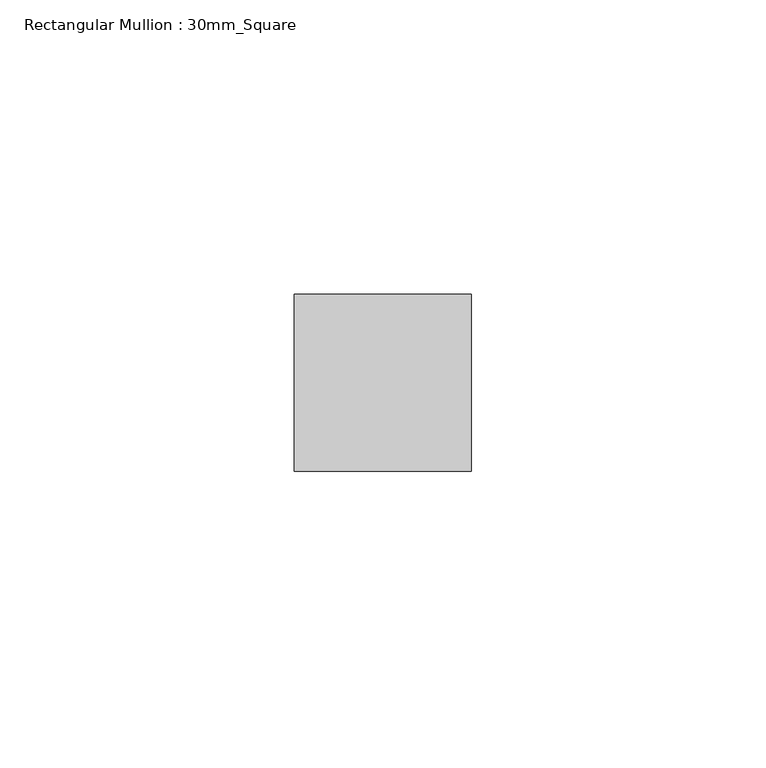
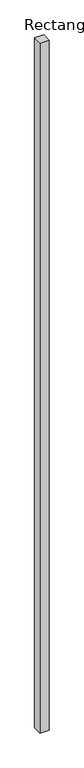
"""IFC4 building model written with IfcOpenShell, lengths in millimetres: member geometry, Rectangular Mullion : 30mm_Square."""

from ifc_helpers import new_model, si_unit, frame, origin, place, context, project, spatial, polyline, outline, extrude, source, transform, mapped, element, save


def rectangular_mullion_30mm_square_b4ecd99e(model_context):
    return source(origin(), model_context, "Body", "SweptSolid", [
        extrude(outline(polyline([(0.0, 15.0), (0.0, -15.0), (-30.0, -15.0), (-30.0, 15.0), (0.0, 15.0)])), frame((0.0, 0.0, -2400.0), z_axis=(0.0, 0.0, 1.0), x_axis=(1.0, 0.0, 0.0)), (0.0, 0.0, 1.0), 2400.0),
    ])


if __name__ == "__main__":
    model = new_model("IFC4")
    model_context = context("Model", 3, world=origin())
    ifc_project = project(units=[si_unit("LENGTHUNIT", "METRE", prefix="MILLI")], contexts=[model_context])
    site = spatial("IfcSite", under=ifc_project)
    building = spatial("IfcBuilding", under=site)
    placement = place(None, origin())
    rectangular_mullion_30mm_square_shape = rectangular_mullion_30mm_square_b4ecd99e(model_context)
    element("IfcMember", 1, ObjectType="Rectangular Mullion : 30mm_Square", at=placement, inside=building, context=model_context, shape_type="MappedRepresentation", body=[
        mapped(rectangular_mullion_30mm_square_shape, transform((0.0, 0.0, 0.0), x_axis=(1.0, 0.0, 0.0), y_axis=(0.0, 1.0, 0.0), z_axis=(0.0, 0.0, 1.0))),
    ])
    save(model, "model.ifc")

# Revit data of these elements
# Type "Rectangular Mullion : 30mm_Square"
#   Keynote = "H11"
#   built-in parameter 1007304 = 0.0984252 (stored number, unit not read)
#   built-in parameter 1007301 = 0.0492126 (stored number, unit not read)
#   built-in parameter 1007300 = 0.0492126 (stored number, unit not read)
# Element 1 (IfcMember, "Rectangular Mullion : 30mm_Square")
#   Materials on its faces: "Aluminium"
# Materials
#   "Aluminium": class "Metal", colour RGB 247 247 247, transparency 0, Description = "Aluminium 6061", Cost = 0
